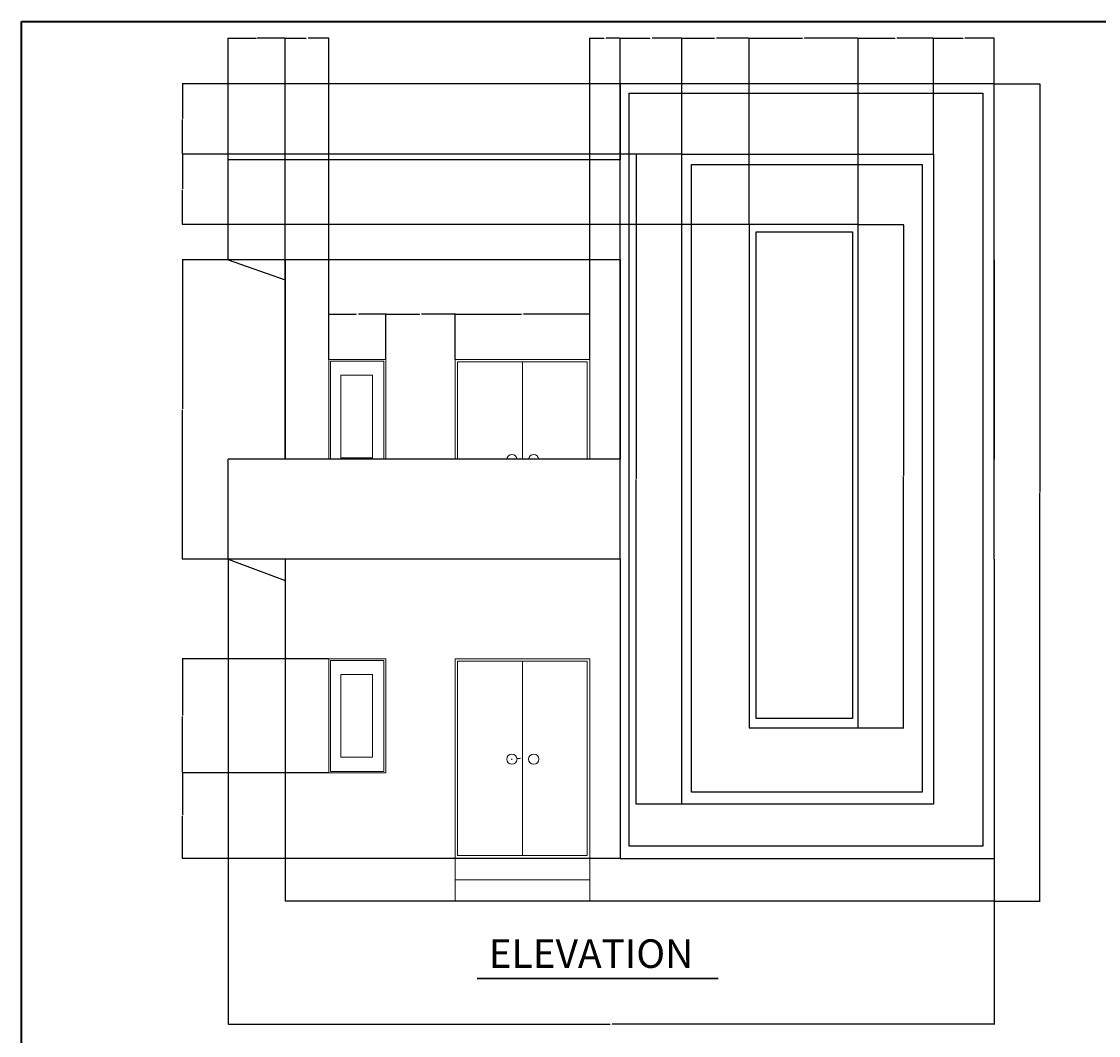
# Model space of a CAD drawing. Units: inches. Extents: x 2416 to 3391, y 1375 to 2496.
# Tile 4 of 13: x 2416 to 2870, y 2069 to 2496. Entities that reach past the tile are written whole.
import ezdxf

# ---------------------------------------------------------------- set-up
doc = ezdxf.new("R2010")
doc.units = ezdxf.units.IN
for name, color, linetype, lineweight in [('A-ANNO-DIMS', 2, 'Continuous', 18), ('A-ANNO-TITL', 7, 'Continuous', 30), ('A-ANNO-TTLB', 7, 'Continuous', 35), ('A-DOOR', 3, 'Continuous', 20), ('A-ELEV', 7, 'Continuous', 25), ('A-FLOR-STRS', 7, 'Continuous', 20), ('A-GLAZ', 4, 'Continuous', 18)]:
    doc.layers.add(name, color=color, linetype=linetype, lineweight=lineweight)
doc.styles.get("Standard").update_dxf_attribs({"font": 'arial.ttf'})
doc.dimstyles.get("Standard").update_dxf_attribs({"dimtxt": 0.18, "dimasz": 0.18, "dimexe": 0.18, "dimexo": 0.0625, "dimgap": 0.09, "dimtad": 0, "dimtih": 1, "dimtoh": 1, "dimdec": 4, "dimzin": 0, "dimdsep": 46, "dimtxsty": 'Standard', "dimcen": 0.09, "dimadec": 0, "dimazin": 0, "dimtfac": 1, "dimtdec": 4, "dimtofl": 0, "dimtmove": 0, "dimatfit": 3, "dimfxl": 1, "dimtolj": 1, "dimtzin": 0, "dimarcsym": 0})

# ---------------------------------------------------------------- blocks, each defined once
blk = doc.blocks.new('*D63')
at = {"layer": 'A-ANNO-DIMS', "color": 0, "lineweight": -2, "transparency": 16777216}
for p, q in [((2503.44, 2269.8), (2503.44, 2074)), ((2825.94, 2125.8), (2825.94, 2074)), ((2503.62, 2074.18), (2664.3, 2074.18)), ((2825.76, 2074.18), (2665.09, 2074.18))]:
    blk.add_line(p, q, dxfattribs=at)
at = {"layer": 'A-ANNO-DIMS', "color": 0, "transparency": 16777216}
for points in [[(2503.62, 2074.21), (2503.62, 2074.15), (2503.44, 2074.18)], [(2825.76, 2074.21), (2825.76, 2074.15), (2825.94, 2074.18)]]:
    blk.add_solid(points, dxfattribs=at)
at = {"layer": 'Defpoints', "color": 0, "transparency": 16777216}
for p in [(2503.44, 2269.86), (2825.94, 2125.86), (2825.94, 2074.18)]:
    blk.add_point(p, dxfattribs=at)
at = {"layer": 'A-ANNO-DIMS', "color": 0, "transparency": 16777216, "insert": (2664.69, 2074.18), "char_height": 0.18, "attachment_point": 5}
blk.add_mtext('\\A1;322.5', dxfattribs=at)
blk = doc.blocks.new('*D64')
at = {"layer": 'A-ANNO-DIMS', "color": 0, "lineweight": -2, "transparency": 16777216}
for p, q in [((2826, 2469.89), (2845.27, 2469.89)), ((2845.09, 2469.71), (2845.09, 2298.06)), ((2845.09, 2126.04), (2845.09, 2297.69)), ((2826, 2125.86), (2845.27, 2125.86))]:
    blk.add_line(p, q, dxfattribs=at)
at = {"layer": 'A-ANNO-DIMS', "color": 0, "transparency": 16777216}
for points in [[(2845.06, 2469.71), (2845.12, 2469.71), (2845.09, 2469.89)], [(2845.06, 2126.04), (2845.12, 2126.04), (2845.09, 2125.86)]]:
    blk.add_solid(points, dxfattribs=at)
at = {"layer": 'Defpoints', "color": 0, "transparency": 16777216}
for p in [(2825.94, 2469.89), (2845.09, 2469.89), (2825.94, 2125.86)]:
    blk.add_point(p, dxfattribs=at)
at = {"layer": 'A-ANNO-DIMS', "color": 0, "transparency": 16777216, "insert": (2845.09, 2297.87), "char_height": 0.18, "attachment_point": 5}
blk.add_mtext('\\A1;344', dxfattribs=at)
blk = doc.blocks.new('*D65')
at = {"layer": 'A-ANNO-DIMS', "color": 0, "lineweight": -2, "transparency": 16777216}
for p, q in [((2503.44, 2437.92), (2503.44, 2489.22)), ((2503.62, 2489.04), (2515.22, 2489.04)), ((2527.26, 2489.04), (2515.66, 2489.04)), ((2527.44, 2387.49), (2527.44, 2489.22))]:
    blk.add_line(p, q, dxfattribs=at)
at = {"layer": 'A-ANNO-DIMS', "color": 0, "transparency": 16777216}
for points in [[(2503.62, 2489.07), (2503.62, 2489.01), (2503.44, 2489.04)], [(2527.26, 2489.07), (2527.26, 2489.01), (2527.44, 2489.04)]]:
    blk.add_solid(points, dxfattribs=at)
at = {"layer": 'Defpoints', "color": 0, "transparency": 16777216}
for p in [(2527.44, 2489.04), (2503.44, 2437.86), (2527.44, 2387.43)]:
    blk.add_point(p, dxfattribs=at)
at = {"layer": 'A-ANNO-DIMS', "color": 0, "transparency": 16777216, "insert": (2515.44, 2489.04), "char_height": 0.18, "attachment_point": 5}
blk.add_mtext('\\A1;24', dxfattribs=at)
blk = doc.blocks.new('*D66')
at = {"layer": 'A-ANNO-DIMS', "color": 0, "lineweight": -2, "transparency": 16777216}
for p, q in [((2527.44, 2311.92), (2527.44, 2489.22)), ((2527.62, 2489.04), (2536.18, 2489.04)), ((2545.64, 2489.04), (2537.09, 2489.04)), ((2545.82, 2353.92), (2545.82, 2489.22))]:
    blk.add_line(p, q, dxfattribs=at)
at = {"layer": 'A-ANNO-DIMS', "color": 0, "transparency": 16777216}
for points in [[(2527.62, 2489.07), (2527.62, 2489.01), (2527.44, 2489.04)], [(2545.64, 2489.07), (2545.64, 2489.01), (2545.82, 2489.04)]]:
    blk.add_solid(points, dxfattribs=at)
at = {"layer": 'Defpoints', "color": 0, "transparency": 16777216}
for p in [(2545.82, 2489.04), (2545.82, 2353.86), (2527.44, 2311.86)]:
    blk.add_point(p, dxfattribs=at)
at = {"layer": 'A-ANNO-DIMS', "color": 0, "transparency": 16777216, "insert": (2536.63, 2489.04), "char_height": 0.18, "attachment_point": 5}
blk.add_mtext('\\A1;18.376', dxfattribs=at)
blk = doc.blocks.new('*D67')
at = {"layer": 'A-ANNO-DIMS', "color": 0, "lineweight": -2, "transparency": 16777216}
for p, q in [((2545.82, 2353.92), (2545.82, 2373.19)), ((2546, 2373.01), (2557.35, 2373.01)), ((2569.64, 2373.01), (2558.28, 2373.01)), ((2569.82, 2353.92), (2569.82, 2373.19))]:
    blk.add_line(p, q, dxfattribs=at)
at = {"layer": 'A-ANNO-DIMS', "color": 0, "transparency": 16777216}
for points in [[(2546, 2373.04), (2546, 2372.98), (2545.82, 2373.01)], [(2569.64, 2373.04), (2569.64, 2372.98), (2569.82, 2373.01)]]:
    blk.add_solid(points, dxfattribs=at)
at = {"layer": 'Defpoints', "color": 0, "transparency": 16777216}
for p in [(2569.82, 2373.01), (2545.82, 2353.86), (2569.82, 2353.86)]:
    blk.add_point(p, dxfattribs=at)
at = {"layer": 'A-ANNO-DIMS', "color": 0, "transparency": 16777216, "insert": (2557.82, 2373.01), "char_height": 0.18, "attachment_point": 5}
blk.add_mtext('\\A1;23.997', dxfattribs=at)
blk = doc.blocks.new('*D68')
at = {"layer": 'A-ANNO-DIMS', "color": 0, "lineweight": -2, "transparency": 16777216}
for p, q in [((2569.82, 2353.92), (2569.82, 2373.19)), ((2570, 2373.01), (2584.02, 2373.01)), ((2598.83, 2373.01), (2584.81, 2373.01)), ((2599.01, 2353.92), (2599.01, 2373.19))]:
    blk.add_line(p, q, dxfattribs=at)
at = {"layer": 'A-ANNO-DIMS', "color": 0, "transparency": 16777216}
for points in [[(2570, 2373.04), (2570, 2372.98), (2569.82, 2373.01)], [(2598.83, 2373.04), (2598.83, 2372.98), (2599.01, 2373.01)]]:
    blk.add_solid(points, dxfattribs=at)
at = {"layer": 'Defpoints', "color": 0, "transparency": 16777216}
for p in [(2599.01, 2373.01), (2569.82, 2353.86), (2599.01, 2353.86)]:
    blk.add_point(p, dxfattribs=at)
at = {"layer": 'A-ANNO-DIMS', "color": 0, "transparency": 16777216, "insert": (2584.41, 2373.01), "char_height": 0.18, "attachment_point": 5}
blk.add_mtext('\\A1;29.19', dxfattribs=at)
blk = doc.blocks.new('*D69')
at = {"layer": 'A-ANNO-DIMS', "color": 0, "lineweight": -2, "transparency": 16777216}
for p, q in [((2599.01, 2353.92), (2599.01, 2373.19)), ((2599.19, 2373.01), (2626.98, 2373.01)), ((2655.55, 2373.01), (2627.76, 2373.01)), ((2655.73, 2353.92), (2655.73, 2373.19))]:
    blk.add_line(p, q, dxfattribs=at)
at = {"layer": 'A-ANNO-DIMS', "color": 0, "transparency": 16777216}
for points in [[(2599.19, 2373.04), (2599.19, 2372.98), (2599.01, 2373.01)], [(2655.55, 2373.04), (2655.55, 2372.98), (2655.73, 2373.01)]]:
    blk.add_solid(points, dxfattribs=at)
at = {"layer": 'Defpoints', "color": 0, "transparency": 16777216}
for p in [(2655.73, 2373.01), (2599.01, 2353.86), (2655.73, 2353.86)]:
    blk.add_point(p, dxfattribs=at)
at = {"layer": 'A-ANNO-DIMS', "color": 0, "transparency": 16777216, "insert": (2627.37, 2373.01), "char_height": 0.18, "attachment_point": 5}
blk.add_mtext('\\A1;56.72', dxfattribs=at)
blk = doc.blocks.new('*D70')
at = {"layer": 'A-ANNO-DIMS', "color": 0, "lineweight": -2, "transparency": 16777216}
for p, q in [((2655.73, 2353.92), (2655.73, 2489.22)), ((2655.91, 2489.04), (2661.63, 2489.04)), ((2668.26, 2489.04), (2662.54, 2489.04)), ((2668.44, 2395.92), (2668.44, 2489.22))]:
    blk.add_line(p, q, dxfattribs=at)
at = {"layer": 'A-ANNO-DIMS', "color": 0, "transparency": 16777216}
for points in [[(2655.91, 2489.07), (2655.91, 2489.01), (2655.73, 2489.04)], [(2668.26, 2489.07), (2668.26, 2489.01), (2668.44, 2489.04)]]:
    blk.add_solid(points, dxfattribs=at)
at = {"layer": 'Defpoints', "color": 0, "transparency": 16777216}
for p in [(2668.44, 2489.04), (2668.44, 2395.86), (2655.73, 2353.86)]:
    blk.add_point(p, dxfattribs=at)
at = {"layer": 'A-ANNO-DIMS', "color": 0, "transparency": 16777216, "insert": (2662.09, 2489.04), "char_height": 0.18, "attachment_point": 5}
blk.add_mtext('\\A1;12.712', dxfattribs=at)
blk = doc.blocks.new('*D71')
at = {"layer": 'A-ANNO-DIMS', "color": 0, "lineweight": -2, "transparency": 16777216}
for p, q in [((2668.44, 2469.95), (2668.44, 2489.22)), ((2668.62, 2489.04), (2680.96, 2489.04)), ((2694.24, 2489.04), (2681.89, 2489.04)), ((2694.42, 2440.34), (2694.42, 2489.22))]:
    blk.add_line(p, q, dxfattribs=at)
at = {"layer": 'A-ANNO-DIMS', "color": 0, "transparency": 16777216}
for points in [[(2668.62, 2489.07), (2668.62, 2489.01), (2668.44, 2489.04)], [(2694.24, 2489.07), (2694.24, 2489.01), (2694.42, 2489.04)]]:
    blk.add_solid(points, dxfattribs=at)
at = {"layer": 'Defpoints', "color": 0, "transparency": 16777216}
for p in [(2694.42, 2489.04), (2668.44, 2469.89), (2694.42, 2440.28)]:
    blk.add_point(p, dxfattribs=at)
at = {"layer": 'A-ANNO-DIMS', "color": 0, "transparency": 16777216, "insert": (2681.43, 2489.04), "char_height": 0.18, "attachment_point": 5}
blk.add_mtext('\\A1;25.974', dxfattribs=at)
blk = doc.blocks.new('*D72')
at = {"layer": 'A-ANNO-DIMS', "color": 0, "lineweight": -2, "transparency": 16777216}
for p, q in [((2694.42, 2440.34), (2694.42, 2489.22)), ((2694.6, 2489.04), (2708.18, 2489.04)), ((2722.56, 2489.04), (2708.98, 2489.04)), ((2722.74, 2410.7), (2722.74, 2489.22))]:
    blk.add_line(p, q, dxfattribs=at)
at = {"layer": 'A-ANNO-DIMS', "color": 0, "transparency": 16777216}
for points in [[(2694.6, 2489.07), (2694.6, 2489.01), (2694.42, 2489.04)], [(2722.56, 2489.07), (2722.56, 2489.01), (2722.74, 2489.04)]]:
    blk.add_solid(points, dxfattribs=at)
at = {"layer": 'Defpoints', "color": 0, "transparency": 16777216}
for p in [(2722.74, 2489.04), (2694.42, 2440.28), (2722.74, 2410.64)]:
    blk.add_point(p, dxfattribs=at)
at = {"layer": 'A-ANNO-DIMS', "color": 0, "transparency": 16777216, "insert": (2708.58, 2489.04), "char_height": 0.18, "attachment_point": 5}
blk.add_mtext('\\A1;28.33', dxfattribs=at)
blk = doc.blocks.new('*D73')
at = {"layer": 'A-ANNO-DIMS', "color": 0, "lineweight": -2, "transparency": 16777216}
for p, q in [((2722.74, 2410.7), (2722.74, 2489.22)), ((2722.92, 2489.04), (2745.28, 2489.04)), ((2768.44, 2489.04), (2746.08, 2489.04)), ((2768.62, 2410.7), (2768.62, 2489.22))]:
    blk.add_line(p, q, dxfattribs=at)
at = {"layer": 'A-ANNO-DIMS', "color": 0, "transparency": 16777216}
for points in [[(2722.92, 2489.07), (2722.92, 2489.01), (2722.74, 2489.04)], [(2768.44, 2489.07), (2768.44, 2489.01), (2768.62, 2489.04)]]:
    blk.add_solid(points, dxfattribs=at)
at = {"layer": 'Defpoints', "color": 0, "transparency": 16777216}
for p in [(2768.62, 2489.04), (2722.74, 2410.64), (2768.62, 2410.64)]:
    blk.add_point(p, dxfattribs=at)
at = {"layer": 'A-ANNO-DIMS', "color": 0, "transparency": 16777216, "insert": (2745.68, 2489.04), "char_height": 0.18, "attachment_point": 5}
blk.add_mtext('\\A1;45.88', dxfattribs=at)
blk = doc.blocks.new('*D74')
at = {"layer": 'A-ANNO-DIMS', "color": 0, "lineweight": -2, "transparency": 16777216}
for p, q in [((2768.62, 2410.7), (2768.62, 2489.22)), ((2768.8, 2489.04), (2784.11, 2489.04)), ((2800.2, 2489.04), (2784.89, 2489.04)), ((2800.38, 2440.34), (2800.38, 2489.22))]:
    blk.add_line(p, q, dxfattribs=at)
at = {"layer": 'A-ANNO-DIMS', "color": 0, "transparency": 16777216}
for points in [[(2768.8, 2489.07), (2768.8, 2489.01), (2768.62, 2489.04)], [(2800.2, 2489.07), (2800.2, 2489.01), (2800.38, 2489.04)]]:
    blk.add_solid(points, dxfattribs=at)
at = {"layer": 'Defpoints', "color": 0, "transparency": 16777216}
for p in [(2800.38, 2489.04), (2800.38, 2440.28), (2768.62, 2410.64)]:
    blk.add_point(p, dxfattribs=at)
at = {"layer": 'A-ANNO-DIMS', "color": 0, "transparency": 16777216, "insert": (2784.5, 2489.04), "char_height": 0.18, "attachment_point": 5}
blk.add_mtext('\\A1;31.76', dxfattribs=at)
blk = doc.blocks.new('*D75')
at = {"layer": 'A-ANNO-DIMS', "color": 0, "lineweight": -2, "transparency": 16777216}
for p, q in [((2800.38, 2440.34), (2800.38, 2489.22)), ((2800.56, 2489.04), (2812.7, 2489.04)), ((2825.76, 2489.04), (2813.63, 2489.04)), ((2825.94, 2469.95), (2825.94, 2489.22))]:
    blk.add_line(p, q, dxfattribs=at)
at = {"layer": 'A-ANNO-DIMS', "color": 0, "transparency": 16777216}
for points in [[(2800.56, 2489.07), (2800.56, 2489.01), (2800.38, 2489.04)], [(2825.76, 2489.07), (2825.76, 2489.01), (2825.94, 2489.04)]]:
    blk.add_solid(points, dxfattribs=at)
at = {"layer": 'Defpoints', "color": 0, "transparency": 16777216}
for p in [(2825.94, 2489.04), (2825.94, 2469.89), (2800.38, 2440.28)]:
    blk.add_point(p, dxfattribs=at)
at = {"layer": 'A-ANNO-DIMS', "color": 0, "transparency": 16777216, "insert": (2813.16, 2489.04), "char_height": 0.18, "attachment_point": 5}
blk.add_mtext('\\A1;25.564', dxfattribs=at)
blk = doc.blocks.new('*D76')
at = {"layer": 'A-ANNO-DIMS', "color": 0, "lineweight": -2, "transparency": 16777216}
for p, q in [((2545.76, 2179.86), (2484.11, 2179.86)), ((2484.29, 2179.68), (2484.29, 2162.04)), ((2484.29, 2144.04), (2484.29, 2161.68)), ((2527.38, 2143.86), (2484.11, 2143.86))]:
    blk.add_line(p, q, dxfattribs=at)
at = {"layer": 'A-ANNO-DIMS', "color": 0, "transparency": 16777216}
for points in [[(2484.26, 2179.68), (2484.32, 2179.68), (2484.29, 2179.86)], [(2484.26, 2144.04), (2484.32, 2144.04), (2484.29, 2143.86)]]:
    blk.add_solid(points, dxfattribs=at)
at = {"layer": 'Defpoints', "color": 0, "transparency": 16777216}
for p in [(2484.29, 2179.86), (2545.82, 2179.86), (2527.44, 2143.86)]:
    blk.add_point(p, dxfattribs=at)
at = {"layer": 'A-ANNO-DIMS', "color": 0, "transparency": 16777216, "insert": (2484.29, 2161.86), "char_height": 0.18, "attachment_point": 5}
blk.add_mtext('\\A1;36', dxfattribs=at)
blk = doc.blocks.new('*D77')
at = {"layer": 'A-ANNO-DIMS', "color": 0, "lineweight": -2, "transparency": 16777216}
for p, q in [((2545.76, 2227.86), (2484.11, 2227.86)), ((2484.29, 2227.68), (2484.29, 2204.04)), ((2484.29, 2180.04), (2484.29, 2203.68)), ((2545.76, 2179.86), (2484.11, 2179.86))]:
    blk.add_line(p, q, dxfattribs=at)
at = {"layer": 'A-ANNO-DIMS', "color": 0, "transparency": 16777216}
for points in [[(2484.26, 2227.68), (2484.32, 2227.68), (2484.29, 2227.86)], [(2484.26, 2180.04), (2484.32, 2180.04), (2484.29, 2179.86)]]:
    blk.add_solid(points, dxfattribs=at)
at = {"layer": 'Defpoints', "color": 0, "transparency": 16777216}
for p in [(2484.29, 2227.86), (2545.82, 2227.86), (2545.82, 2179.86)]:
    blk.add_point(p, dxfattribs=at)
at = {"layer": 'A-ANNO-DIMS', "color": 0, "transparency": 16777216, "insert": (2484.29, 2203.86), "char_height": 0.18, "attachment_point": 5}
blk.add_mtext('\\A1;48', dxfattribs=at)
blk = doc.blocks.new('*D78')
at = {"layer": 'A-ANNO-DIMS', "color": 0, "lineweight": -2, "transparency": 16777216}
for p, q in [((2503.38, 2395.86), (2484.11, 2395.86)), ((2484.29, 2395.68), (2484.29, 2333.04)), ((2484.29, 2270.04), (2484.29, 2332.68)), ((2503.38, 2269.86), (2484.11, 2269.86))]:
    blk.add_line(p, q, dxfattribs=at)
at = {"layer": 'A-ANNO-DIMS', "color": 0, "transparency": 16777216}
for points in [[(2484.26, 2395.68), (2484.32, 2395.68), (2484.29, 2395.86)], [(2484.26, 2270.04), (2484.32, 2270.04), (2484.29, 2269.86)]]:
    blk.add_solid(points, dxfattribs=at)
at = {"layer": 'Defpoints', "color": 0, "transparency": 16777216}
for p in [(2484.29, 2395.86), (2503.44, 2395.86), (2503.44, 2269.86)]:
    blk.add_point(p, dxfattribs=at)
at = {"layer": 'A-ANNO-DIMS', "color": 0, "transparency": 16777216, "insert": (2484.29, 2332.86), "char_height": 0.18, "attachment_point": 5}
blk.add_mtext('\\A1;126', dxfattribs=at)
blk = doc.blocks.new('*D79')
at = {"layer": 'A-ANNO-DIMS', "color": 0, "lineweight": -2, "transparency": 16777216}
for p, q in [((2668.38, 2469.89), (2484.11, 2469.89)), ((2484.29, 2469.71), (2484.29, 2455.26)), ((2484.29, 2440.46), (2484.29, 2454.9)), ((2694.35, 2440.28), (2484.11, 2440.28))]:
    blk.add_line(p, q, dxfattribs=at)
at = {"layer": 'A-ANNO-DIMS', "color": 0, "transparency": 16777216}
for points in [[(2484.26, 2469.71), (2484.32, 2469.71), (2484.29, 2469.89)], [(2484.26, 2440.46), (2484.32, 2440.46), (2484.29, 2440.28)]]:
    blk.add_solid(points, dxfattribs=at)
at = {"layer": 'Defpoints', "color": 0, "transparency": 16777216}
for p in [(2484.29, 2469.89), (2668.44, 2469.89), (2694.42, 2440.28)]:
    blk.add_point(p, dxfattribs=at)
at = {"layer": 'A-ANNO-DIMS', "color": 0, "transparency": 16777216, "insert": (2484.29, 2455.08), "char_height": 0.18, "attachment_point": 5}
blk.add_mtext('\\A1;29.61', dxfattribs=at)
blk = doc.blocks.new('*D80')
at = {"layer": 'A-ANNO-DIMS', "color": 0, "lineweight": -2, "transparency": 16777216}
for p, q in [((2694.35, 2440.28), (2484.11, 2440.28)), ((2484.29, 2440.1), (2484.29, 2425.64)), ((2484.29, 2410.82), (2484.29, 2425.27)), ((2722.68, 2410.64), (2484.11, 2410.64))]:
    blk.add_line(p, q, dxfattribs=at)
at = {"layer": 'A-ANNO-DIMS', "color": 0, "transparency": 16777216}
for points in [[(2484.26, 2440.1), (2484.32, 2440.1), (2484.29, 2440.28)], [(2484.26, 2410.82), (2484.32, 2410.82), (2484.29, 2410.64)]]:
    blk.add_solid(points, dxfattribs=at)
at = {"layer": 'Defpoints', "color": 0, "transparency": 16777216}
for p in [(2484.29, 2440.28), (2694.42, 2440.28), (2722.74, 2410.64)]:
    blk.add_point(p, dxfattribs=at)
at = {"layer": 'A-ANNO-DIMS', "color": 0, "transparency": 16777216, "insert": (2484.29, 2425.46), "char_height": 0.18, "attachment_point": 5}
blk.add_mtext('\\A1;29.64', dxfattribs=at)
blk = doc.blocks.new('*D81')
at = {"layer": 'A-ANNO-DIMS', "color": 0, "lineweight": -2, "transparency": 16777216}
for p, q in [((2768.68, 2410.64), (2787.95, 2410.64)), ((2787.77, 2410.46), (2787.77, 2304.96)), ((2787.77, 2199.09), (2787.77, 2304.59)), ((2768.68, 2198.91), (2787.95, 2198.91))]:
    blk.add_line(p, q, dxfattribs=at)
at = {"layer": 'A-ANNO-DIMS', "color": 0, "transparency": 16777216}
for points in [[(2787.74, 2410.46), (2787.8, 2410.46), (2787.77, 2410.64)], [(2787.74, 2199.09), (2787.8, 2199.09), (2787.77, 2198.91)]]:
    blk.add_solid(points, dxfattribs=at)
at = {"layer": 'Defpoints', "color": 0, "transparency": 16777216}
for p in [(2768.62, 2410.64), (2768.62, 2198.91), (2787.77, 2198.91)]:
    blk.add_point(p, dxfattribs=at)
at = {"layer": 'A-ANNO-DIMS', "color": 0, "transparency": 16777216, "insert": (2787.77, 2304.77), "char_height": 0.18, "attachment_point": 5}
blk.add_mtext('\\A1;211.73', dxfattribs=at)
blk = doc.blocks.new('*D82')
at = {"layer": 'A-ANNO-DIMS', "color": 0, "lineweight": -2, "transparency": 16777216}
for p, q in [((2694.35, 2440.28), (2675.09, 2440.28)), ((2675.27, 2440.1), (2675.27, 2303.7)), ((2675.27, 2166.93), (2675.27, 2303.33)), ((2694.35, 2166.75), (2675.09, 2166.75))]:
    blk.add_line(p, q, dxfattribs=at)
at = {"layer": 'A-ANNO-DIMS', "color": 0, "transparency": 16777216}
for points in [[(2675.24, 2440.1), (2675.3, 2440.1), (2675.27, 2440.28)], [(2675.24, 2166.93), (2675.3, 2166.93), (2675.27, 2166.75)]]:
    blk.add_solid(points, dxfattribs=at)
at = {"layer": 'Defpoints', "color": 0, "transparency": 16777216}
for p in [(2675.27, 2440.28), (2694.42, 2440.28), (2694.42, 2166.75)]:
    blk.add_point(p, dxfattribs=at)
at = {"layer": 'A-ANNO-DIMS', "color": 0, "transparency": 16777216, "insert": (2675.27, 2303.52), "char_height": 0.18, "attachment_point": 5}
blk.add_mtext('\\A1;273.5', dxfattribs=at)
blk = doc.blocks.new('*D88')
at = {"layer": 'A-ANNO-DIMS', "color": 0, "lineweight": -2, "transparency": 16777216}
for p, q in [((2622.82, 2185.68), (2623, 2185.68)), ((2622.91, 2185.59), (2622.91, 2185.77)), ((2626.36, 2185.98), (2625.24, 2185.88))]:
    blk.add_line(p, q, dxfattribs=at)
at = {"layer": 'A-ANNO-DIMS', "color": 0, "transparency": 16777216}
blk.add_solid([(2625.24, 2185.91), (2625.24, 2185.85), (2625.06, 2185.87)], dxfattribs=at)
at = {"layer": 'Defpoints', "color": 0, "transparency": 16777216}
for p in [(2620.75, 2185.49), (2625.06, 2185.87)]:
    blk.add_point(p, dxfattribs=at)
at = {"layer": 'A-ANNO-DIMS', "color": 0, "transparency": 16777216, "insert": (2627.04, 2185.98), "char_height": 0.18, "attachment_point": 5}
blk.add_mtext('\\A1;2X ∅4.326', dxfattribs=at)

msp = doc.modelspace()

# ---------------------------------------------------------------- linework, layer by layer
at = {"layer": 'A-ANNO-TITL'}
msp.add_line((2608.3129, 2093.3344), (2709.7105, 2093.3344), dxfattribs=at)
at = {"layer": 'A-ANNO-TTLB'}
msp.add_lwpolyline([(2416.4678, 2496.0939), (3391.2022, 2496.0939), (3391.2022, 1375.1104), (2416.4678, 1375.1104)], close=True, dxfattribs=at)
at = {"layer": 'A-DOOR'}
for p, q in [((2599.0081, 2353.8608), (2599.0081, 2311.8608)), ((2655.7305, 2353.8608), (2599.0081, 2353.8608)), ((2599.0081, 2353.8608), (2599.0081, 2311.8608)), ((2655.7305, 2353.8608), (2599.0081, 2353.8608)), ((2655.7305, 2353.8608), (2655.7305, 2311.8608)), ((2655.7305, 2353.8608), (2655.7305, 2311.8608)), ((2627.3007, 2352.8759), (2627.3007, 2311.8608)), ((2599.0081, 2227.8608), (2599.0081, 2143.8608)), ((2655.7305, 2227.8608), (2599.0081, 2227.8608)), ((2627.3007, 2226.8759), (2627.3007, 2145.071)), ((2655.7305, 2227.8608), (2655.7305, 2143.8608))]:
    msp.add_line(p, q, dxfattribs=at)
msp.add_lwpolyline([(2599.9818, 2311.8608), (2599.9818, 2352.8759), (2654.6195, 2352.8759), (2654.6195, 2311.8608)], dxfattribs=at)
msp.add_lwpolyline([(2599.9818, 2226.8759), (2654.6195, 2226.8759), (2654.6195, 2145.071), (2599.9818, 2145.071)], close=True, dxfattribs=at)
for centre in [(2622.9077, 2185.6767), (2632.0851, 2185.6767)]:
    msp.add_circle(centre, 2.1629, dxfattribs=at)
for centre in [(2622.9077, 2311.6767), (2632.0851, 2311.6767)]:
    msp.add_arc(centre, 2.1629, 4.882603, 175.117397, dxfattribs=at)
at = {"layer": 'A-ELEV'}
for p, q in [((2825.9424, 2469.887), (2668.4424, 2469.887)), ((2668.4424, 2469.887), (2668.4424, 2437.8608)), ((2825.9424, 2437.8608), (2825.9424, 2469.887)), ((2668.4424, 2437.8608), (2503.4424, 2437.8608)), ((2503.4424, 2395.8608), (2503.4424, 2437.8608)), ((2668.4424, 2269.8608), (2668.4424, 2437.8608)), ((2825.9424, 2269.8608), (2825.9424, 2437.8608)), ((2668.4424, 2395.8608), (2503.4424, 2395.8608)), ((2503.4424, 2395.8608), (2527.4424, 2387.429)), ((2527.4424, 2395.8608), (2527.4424, 2311.8608)), ((2668.4424, 2395.8608), (2668.4424, 2311.8608)), ((2825.9424, 2395.8608), (2825.9424, 2311.8608)), ((2668.4424, 2311.8608), (2503.4424, 2311.8608)), ((2503.4424, 2269.8608), (2503.4424, 2311.8608)), ((2668.4424, 2269.8608), (2503.4424, 2269.8608)), ((2503.4424, 2269.8608), (2527.4424, 2260.8608)), ((2527.4424, 2269.8608), (2527.4424, 2125.8608)), ((2527.4424, 2269.8608), (2527.4424, 2251.8608)), ((2668.4424, 2269.8608), (2668.4424, 2143.8608)), ((2825.9424, 2269.8608), (2825.9424, 2125.8608)), ((2825.9424, 2269.8608), (2825.9424, 2251.8608)), ((2668.4424, 2143.8608), (2527.4424, 2143.8608)), ((2668.4424, 2143.8608), (2825.9424, 2143.8608)), ((2825.9424, 2125.8608), (2527.4424, 2125.8608))]:
    msp.add_line(p, q, dxfattribs=at)
for points in [[(2672.2026, 2465.9119), (2821.223, 2465.9119), (2821.223, 2149.0349), (2672.2026, 2149.0349)], [(2694.4163, 2440.2765), (2800.3785, 2440.2765), (2800.3785, 2166.7537), (2694.4163, 2166.7537)], [(2698.5392, 2435.8809), (2795.6258, 2435.8809), (2795.6258, 2171.7713), (2698.5392, 2171.7713)], [(2768.6209, 2410.6371), (2722.744, 2410.6371), (2722.744, 2198.9095), (2768.6209, 2198.9095)], [(2725.7851, 2407.5924), (2766.319, 2407.5924), (2766.319, 2202.7738), (2725.7851, 2202.7738)]]:
    msp.add_lwpolyline(points, close=True, dxfattribs=at)
at = {"layer": 'A-FLOR-STRS'}
for p, q in [((2599.0081, 2143.8608), (2599.0081, 2125.8608)), ((2655.7305, 2143.8608), (2655.7305, 2125.8608)), ((2655.7305, 2134.8608), (2599.0081, 2134.8608)), ((2655.7305, 2125.8608), (2655.7305, 2134.8608))]:
    msp.add_line(p, q, dxfattribs=at)
at = {"layer": 'A-GLAZ'}
for p, q in [((2545.8186, 2353.8608), (2545.8186, 2311.8608)), ((2569.8155, 2353.8608), (2545.8186, 2353.8608)), ((2545.8186, 2353.8608), (2545.8186, 2311.8608)), ((2569.8155, 2353.8608), (2545.8186, 2353.8608)), ((2569.8155, 2353.8608), (2569.8155, 2311.8608)), ((2569.8155, 2353.8608), (2569.8155, 2311.8608)), ((2545.8186, 2227.8608), (2545.8186, 2179.8608)), ((2569.8155, 2227.8608), (2545.8186, 2227.8608)), ((2569.8155, 2227.8608), (2569.8155, 2179.8608)), ((2569.8155, 2179.8608), (2545.8186, 2179.8608))]:
    msp.add_line(p, q, dxfattribs=at)
msp.add_lwpolyline([(2546.5017, 2311.8608), (2546.5017, 2353.1409), (2568.9368, 2353.1409), (2568.9368, 2311.8608)], dxfattribs=at)
for points in [[(2550.928, 2347.3074), (2564.1934, 2347.3074), (2564.1934, 2312.4761), (2550.928, 2312.4761)], [(2546.5017, 2227.1409), (2568.9368, 2227.1409), (2568.9368, 2180.5158), (2546.5017, 2180.5158)], [(2550.928, 2221.3074), (2564.1934, 2221.3074), (2564.1934, 2186.4761), (2550.928, 2186.4761)]]:
    msp.add_lwpolyline(points, close=True, dxfattribs=at)

# ---------------------------------------------------------------- texts
at = {"layer": 'A-ANNO-TITL', "insert": (2613.1221, 2109.8305), "char_height": 12, "attachment_point": 1}
msp.add_mtext_dynamic_manual_height_columns('ELEVATION', width=220.225454, gutter_width=12.5, heights=[0], dxfattribs=at)

# ---------------------------------------------------------------- dimensions: what is measured, and where the dimension line sits
at = {"layer": 'A-ANNO-DIMS'}
for base, p1, p2, override, picture, middle in [((2527.4424, 2489.037), (2503.4424, 2437.8608), (2527.4424, 2387.429), {"dimdec": 0, "dimlfac": 1, "dimrnd": 0, "dimzin": 0, "dimdsep": 46, "dimlunit": 2}, '*D65', (2515.4424, 2489.037)), ((2545.8186, 2489.037), (2527.4424, 2311.8608), (2545.8186, 2353.8608), {"dimdec": 3, "dimlfac": 1, "dimrnd": 0, "dimzin": 0, "dimdsep": 46, "dimlunit": 2}, '*D66', (2536.6305, 2489.037)), ((2668.4424, 2489.037), (2655.7305, 2353.8608), (2668.4424, 2395.8608), {"dimdec": 3, "dimlfac": 1, "dimrnd": 0, "dimzin": 0, "dimdsep": 46, "dimlunit": 2}, '*D70', (2662.0864, 2489.037)), ((2694.4163, 2489.037), (2668.4424, 2469.887), (2694.4163, 2440.2765), {"dimdec": 3, "dimlfac": 1, "dimrnd": 0, "dimzin": 0, "dimdsep": 46, "dimlunit": 2}, '*D71', (2681.4293, 2489.037)), ((2722.744, 2489.037), (2694.4163, 2440.2765), (2722.744, 2410.6371), {"dimdec": 2, "dimlfac": 1, "dimrnd": 0, "dimzin": 0, "dimdsep": 46, "dimlunit": 2}, '*D72', (2708.5802, 2489.037)), ((2768.6209, 2489.037), (2722.744, 2410.6371), (2768.6209, 2410.6371), {"dimdec": 2, "dimlfac": 1, "dimrnd": 0, "dimzin": 0, "dimdsep": 46, "dimlunit": 2}, '*D73', (2745.6825, 2489.037)), ((2800.3785, 2489.037), (2768.6209, 2410.6371), (2800.3785, 2440.2765), {"dimdec": 2, "dimlfac": 1, "dimrnd": 0, "dimzin": 0, "dimdsep": 46, "dimlunit": 2}, '*D74', (2784.4997, 2489.037)), ((2825.9424, 2489.037), (2800.3785, 2440.2765), (2825.9424, 2469.887), {"dimdec": 3, "dimlfac": 1, "dimrnd": 0, "dimzin": 0, "dimdsep": 46, "dimlunit": 2}, '*D75', (2813.1604, 2489.037)), ((2569.8155, 2373.0108), (2545.8186, 2353.8608), (2569.8155, 2353.8608), {"dimdec": 3, "dimlfac": 1, "dimrnd": 0, "dimzin": 0, "dimdsep": 46, "dimlunit": 2}, '*D67', (2557.8171, 2373.0108)), ((2599.0081, 2373.0108), (2569.8155, 2353.8608), (2599.0081, 2353.8608), {"dimdec": 2, "dimlfac": 1, "dimrnd": 0, "dimzin": 0, "dimdsep": 46, "dimlunit": 2}, '*D68', (2584.4118, 2373.0108)), ((2655.7305, 2373.0108), (2599.0081, 2353.8608), (2655.7305, 2353.8608), {"dimdec": 2, "dimlfac": 1, "dimrnd": 0, "dimzin": 0, "dimdsep": 46, "dimlunit": 2}, '*D69', (2627.3693, 2373.0108)), ((2825.9424, 2074.1844), (2503.4424, 2269.8608), (2825.9424, 2125.8608), {"dimdec": 1, "dimlfac": 1, "dimrnd": 0, "dimzin": 0, "dimdsep": 46, "dimlunit": 2}, '*D63', (2664.6924, 2074.1844))]:
    dim = msp.add_linear_dim(base=base, p1=p1, p2=p2, dimstyle='Standard', override=override, dxfattribs=at)
    dim.commit()
    dim.dimension.update_dxf_attribs({"geometry": picture, "text_midpoint": middle})
for base, p1, p2, angle, override, picture, middle in [((2484.2924, 2469.887), (2694.4163, 2440.2765), (2668.4424, 2469.887), 90, {"dimdec": 2, "dimlfac": 1, "dimrnd": 0, "dimzin": 0, "dimdsep": 46, "dimlunit": 2}, '*D79', (2484.2924, 2455.0817)), ((2845.0924, 2469.887), (2825.9424, 2125.8608), (2825.9424, 2469.887), 90, {"dimdec": 0, "dimlfac": 1, "dimrnd": 0, "dimzin": 0, "dimdsep": 46, "dimlunit": 2}, '*D64', (2845.0924, 2297.8739)), ((2484.2924, 2440.2765), (2722.744, 2410.6371), (2694.4163, 2440.2765), 90, {"dimdec": 2, "dimlfac": 1, "dimrnd": 0, "dimzin": 0, "dimdsep": 46, "dimlunit": 2}, '*D80', (2484.2924, 2425.4568)), ((2675.2663, 2440.2765), (2694.4163, 2166.7537), (2694.4163, 2440.2765), 90, {"dimdec": 1, "dimlfac": 1, "dimrnd": 0, "dimzin": 0, "dimdsep": 46, "dimlunit": 2}, '*D82', (2675.2663, 2303.5151)), ((2787.7709, 2198.9095), (2768.6209, 2410.6371), (2768.6209, 2198.9095), 270, {"dimdec": 2, "dimlfac": 1, "dimrnd": 0, "dimzin": 0, "dimdsep": 46, "dimlunit": 2}, '*D81', (2787.7709, 2304.7733)), ((2484.2924, 2395.8608), (2503.4424, 2269.8608), (2503.4424, 2395.8608), 90, {"dimdec": 0, "dimlfac": 1, "dimrnd": 0, "dimzin": 0, "dimdsep": 46, "dimlunit": 2}, '*D78', (2484.2924, 2332.8608)), ((2484.2924, 2227.8608), (2545.8186, 2179.8608), (2545.8186, 2227.8608), 90, {"dimdec": 0, "dimlfac": 1, "dimrnd": 0, "dimzin": 0, "dimdsep": 46, "dimlunit": 2}, '*D77', (2484.2924, 2203.8608)), ((2484.2924, 2179.8608), (2527.4424, 2143.8608), (2545.8186, 2179.8608), 90, {"dimdec": 0, "dimlfac": 1, "dimrnd": 0, "dimzin": 0, "dimdsep": 46, "dimlunit": 2}, '*D76', (2484.2924, 2161.8608))]:
    dim = msp.add_linear_dim(base=base, p1=p1, p2=p2, angle=angle, dimstyle='Standard', override=override, dxfattribs=at)
    dim.commit()
    dim.dimension.update_dxf_attribs({"geometry": picture, "text_midpoint": middle})
dim = msp.add_diameter_dim_2p(p1=(2620.753, 2185.4879), p2=(2625.0623, 2185.8655), text='2X <>', dimstyle='Standard', override={"dimdec": 3, "dimlfac": 1, "dimrnd": 0, "dimzin": 0, "dimdsep": 46, "dimlunit": 2}, dxfattribs=at)
dim.commit()
dim.dimension.update_dxf_attribs({"geometry": '*D88', "text_midpoint": (2626.3551, 2185.9787), "dimtype": 163})

doc.saveas('drawing.dxf')
